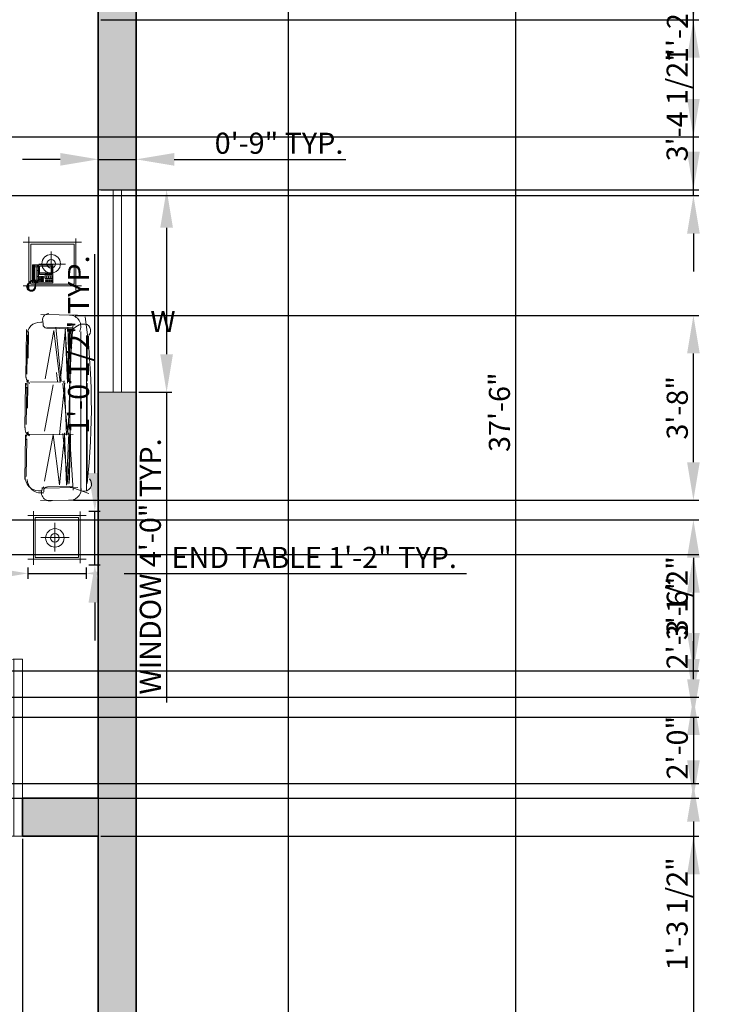
# Model space of a CAD drawing. Units: inches. Extents: x 2265 to 2807, y 1544 to 2401.
# Tile 8 of 9: x 2643 to 2807, y 1890 to 2124. Entities that reach past the tile are written whole.
import ezdxf

# ---------------------------------------------------------------- set-up
doc = ezdxf.new("R2010")
doc.units = ezdxf.units.IN
for name, color, linetype, lineweight in [('A-ANNO-DIMS', 2, 'Continuous', 18), ('A-ANNO-TEXT', 7, 'Continuous', 18), ('A-DOOR', 3, 'Continuous', 18), ('A-GLAZ', 4, 'Continuous', 18), ('A-WALL', 7, 'Continuous', 35), ('A-WALL-PATT', 18, 'Continuous', 13), ('C-PROP', 7, 'Continuous', 25), ('Furniture', 161, 'Continuous', 15)]:
    doc.layers.add(name, color=color, linetype=linetype, lineweight=lineweight)
doc.styles.add('ARIAL', font='times.ttf', dxfattribs={"height": 5})
doc.styles.get("Standard").update_dxf_attribs({"font": 'arial.ttf', "height": 5})
doc.dimstyles.new('ISO-25', dxfattribs={"dimtxt": 5, "dimasz": 9, "dimexe": 1.25, "dimexo": 0.625, "dimtad": 1, "dimlunit": 3, "dimtxsty": 'Standard', "dimcen": 2.5, "dimadec": 0, "dimazin": 0, "dimtfac": 1, "dimtmove": 0, "dimatfit": 3, "dimfxl": 1, "dimarcsym": 0})

# ---------------------------------------------------------------- blocks, each defined once
blk = doc.blocks.new('*D6')
at = {"layer": 'A-ANNO-DIMS', "color": 0, "lineweight": -2, "transparency": 16777216}
for p, q in [((2707.73, 2255.73), (2762.29, 2255.73)), ((2761.04, 2246.73), (2761.04, 1814.73)), ((2707.73, 1805.73), (2762.29, 1805.73))]:
    blk.add_line(p, q, dxfattribs=at)
at = {"layer": 'A-ANNO-DIMS', "color": 0, "lineweight": 100, "transparency": 16777216}
for points in [[(2759.54, 2246.73), (2762.54, 2246.73), (2761.04, 2255.73)], [(2759.54, 1814.73), (2762.54, 1814.73), (2761.04, 1805.73)]]:
    blk.add_solid(points, dxfattribs=at)
at = {"layer": 'Defpoints', "color": 0, "lineweight": 100, "transparency": 16777216}
for p in [(2707.1, 2255.73), (2707.1, 1805.73), (2761.04, 1805.73)]:
    blk.add_point(p, dxfattribs=at)
at = {"layer": 'A-ANNO-DIMS', "color": 0, "transparency": 16777216, "insert": (2757.86, 2030.73), "char_height": 5, "attachment_point": 5, "rotation": 90}
blk.add_mtext('37\'-6"', dxfattribs=at)
blk = doc.blocks.new('GLAZING-48IN')
for p, q in [((48, 9), (0, 9)), ((0, 5.5), (48, 5.5)), ((0, 5.5), (48, 5.5)), ((0, 3.5), (48, 3.5)), ((0, 0), (48, 0))]:
    blk.add_line(p, q)
blk = doc.blocks.new('END-TABLE')
for p, q in [((1.35, 12.69), (1.35, 0)), ((12.46, 0.37), (12.46, 12.6)), ((13.82, 11.62), (0, 11.62)), ((1.77, 11.2), (1.77, 1.7)), ((12.04, 11.2), (1.77, 11.2)), ((12.04, 1.7), (12.04, 11.2)), ((0, 1.28), (13.82, 1.28)), ((1.77, 1.7), (12.04, 1.7))]:
    blk.add_line(p, q)
blk = doc.blocks.new('DOOR-SWING-42IN')
for p, q in [((40, 41.95), (40, 0)), ((42, 0), (0, 0))]:
    blk.add_line(p, q)
blk.add_arc((42, 0), 42, 90, 180)
blk = doc.blocks.new('*D19')
at = {"layer": 'A-ANNO-DIMS', "color": 0, "lineweight": -2, "transparency": 16777216}
for p, q in [((2671.73, 2083.44), (2679.55, 2083.44)), ((2678.3, 2074.44), (2678.3, 2044.44)), ((2671.73, 2035.44), (2679.55, 2035.44)), ((2678.3, 2035.44), (2678.3, 1961.91))]:
    blk.add_line(p, q, dxfattribs=at)
at = {"layer": 'A-ANNO-DIMS', "color": 0, "lineweight": 100, "transparency": 16777216}
for points in [[(2676.8, 2074.44), (2679.8, 2074.44), (2678.3, 2083.44)], [(2676.8, 2044.44), (2679.8, 2044.44), (2678.3, 2035.44)]]:
    blk.add_solid(points, dxfattribs=at)
at = {"layer": 'Defpoints', "color": 0, "lineweight": 100, "transparency": 16777216}
for p in [(2671.1, 2083.44), (2671.1, 2035.44), (2678.3, 2035.44)]:
    blk.add_point(p, dxfattribs=at)
at = {"layer": 'A-ANNO-DIMS', "color": 0, "transparency": 16777216, "insert": (2675.09, 1994.17), "char_height": 5, "attachment_point": 5, "rotation": 90}
blk.add_mtext('WINDOW 4\'-0" TYP.', dxfattribs=at)
blk = doc.blocks.new('*D20')
at = {"layer": 'A-ANNO-DIMS', "color": 0, "lineweight": -2, "transparency": 16777216}
for p, q in [((2653.1, 2090.64), (2644.1, 2090.64)), ((2662.1, 2084.06), (2662.1, 2091.89)), ((2662.1, 2090.64), (2671.1, 2090.64)), ((2671.1, 2084.06), (2671.1, 2091.89)), ((2680.1, 2090.64), (2720.83, 2090.64))]:
    blk.add_line(p, q, dxfattribs=at)
at = {"layer": 'A-ANNO-DIMS', "color": 0, "lineweight": 100, "transparency": 16777216}
for points in [[(2653.1, 2092.14), (2653.1, 2089.14), (2662.1, 2090.64)], [(2680.1, 2092.14), (2680.1, 2089.14), (2671.1, 2090.64)]]:
    blk.add_solid(points, dxfattribs=at)
at = {"layer": 'Defpoints', "color": 0, "lineweight": 100, "transparency": 16777216}
for p in [(2671.1, 2090.64), (2662.1, 2083.44), (2671.1, 2083.44)]:
    blk.add_point(p, dxfattribs=at)
at = {"layer": 'A-ANNO-DIMS', "color": 0, "transparency": 16777216, "insert": (2704.96, 2093.81), "char_height": 5, "attachment_point": 5}
blk.add_mtext('0\'-9" TYP.', dxfattribs=at)
blk = doc.blocks.new('*D29')
at = {"layer": 'A-ANNO-DIMS', "color": 0, "lineweight": -2, "transparency": 16777216}
for p, q in [((2645.38, 1993.96), (2645.38, 1991.27)), ((2659.2, 1993.96), (2659.2, 1991.27)), ((2636.38, 1992.52), (2627.38, 1992.52)), ((2645.38, 1992.52), (2659.2, 1992.52)), ((2668.2, 1992.52), (2749.43, 1992.52))]:
    blk.add_line(p, q, dxfattribs=at)
at = {"layer": 'A-ANNO-DIMS', "color": 0, "lineweight": 100, "transparency": 16777216}
for points in [[(2636.38, 1994.02), (2636.38, 1991.02), (2645.38, 1992.52)], [(2668.2, 1994.02), (2668.2, 1991.02), (2659.2, 1992.52)]]:
    blk.add_solid(points, dxfattribs=at)
at = {"layer": 'Defpoints', "color": 0, "lineweight": 100, "transparency": 16777216}
for p in [(2645.38, 1994.59), (2659.2, 1994.59), (2659.2, 1992.52)]:
    blk.add_point(p, dxfattribs=at)
at = {"layer": 'A-ANNO-DIMS', "color": 0, "transparency": 16777216, "insert": (2713.31, 1995.65), "char_height": 5, "attachment_point": 5}
blk.add_mtext('END TABLE 1\'-2" TYP.', dxfattribs=at)
blk = doc.blocks.new('*D30')
at = {"layer": 'A-ANNO-DIMS', "color": 0, "lineweight": -2, "transparency": 16777216}
for p, q in [((2661.28, 2016.28), (2661.28, 2068.19)), ((2659.83, 2007.28), (2662.53, 2007.28)), ((2661.28, 1994.59), (2661.28, 2007.28)), ((2659.83, 1994.59), (2662.53, 1994.59)), ((2661.28, 1985.59), (2661.28, 1976.59))]:
    blk.add_line(p, q, dxfattribs=at)
at = {"layer": 'A-ANNO-DIMS', "color": 0, "lineweight": 100, "transparency": 16777216}
for points in [[(2659.78, 2016.28), (2662.78, 2016.28), (2661.28, 2007.28)], [(2659.78, 1985.59), (2662.78, 1985.59), (2661.28, 1994.59)]]:
    blk.add_solid(points, dxfattribs=at)
at = {"layer": 'Defpoints', "color": 0, "lineweight": 100, "transparency": 16777216}
for p in [(2659.2, 2007.28), (2661.28, 2007.28), (2659.2, 1994.59)]:
    blk.add_point(p, dxfattribs=at)
at = {"layer": 'A-ANNO-DIMS', "color": 0, "transparency": 16777216, "insert": (2658.07, 2046.74), "char_height": 5, "attachment_point": 5, "rotation": 90}
blk.add_mtext('1\'-0 1/2" TYP.', dxfattribs=at)
blk = doc.blocks.new('*D35')
at = {"layer": 'A-ANNO-DIMS', "color": 0, "lineweight": -2, "transparency": 16777216}
for p, q in [((2581.1, 2123.11), (2581.1, 1546.93)), ((2662.1, 2123.11), (2662.1, 1546.93)), ((2590.1, 1548.18), (2653.1, 1548.18))]:
    blk.add_line(p, q, dxfattribs=at)
at = {"layer": 'A-ANNO-DIMS', "color": 0, "lineweight": 100, "transparency": 16777216}
for points in [[(2590.1, 1549.68), (2590.1, 1546.68), (2581.1, 1548.18)], [(2653.1, 1549.68), (2653.1, 1546.68), (2662.1, 1548.18)]]:
    blk.add_solid(points, dxfattribs=at)
at = {"layer": 'Defpoints', "color": 0, "lineweight": 100, "transparency": 16777216}
for p in [(2581.1, 2123.73), (2662.1, 2123.73), (2662.1, 1548.18)]:
    blk.add_point(p, dxfattribs=at)
at = {"layer": 'A-ANNO-DIMS', "color": 0, "transparency": 16777216, "insert": (2621.6, 1551.36), "char_height": 5, "attachment_point": 5}
blk.add_mtext('6\'-9"', dxfattribs=at)
blk = doc.blocks.new('*D36')
at = {"layer": 'A-ANNO-DIMS', "color": 0, "lineweight": -2, "transparency": 16777216}
for p, q in [((2662.73, 2246.73), (2804.46, 2246.73)), ((2803.21, 2237.73), (2803.21, 2132.73)), ((2662.73, 2123.73), (2804.46, 2123.73))]:
    blk.add_line(p, q, dxfattribs=at)
at = {"layer": 'A-ANNO-DIMS', "color": 0, "lineweight": 100, "transparency": 16777216}
for points in [[(2801.71, 2237.73), (2804.71, 2237.73), (2803.21, 2246.73)], [(2801.71, 2132.73), (2804.71, 2132.73), (2803.21, 2123.73)]]:
    blk.add_solid(points, dxfattribs=at)
at = {"layer": 'Defpoints', "color": 0, "lineweight": 100, "transparency": 16777216}
for p in [(2662.1, 2246.73), (2662.1, 2123.73), (2803.21, 2123.73)]:
    blk.add_point(p, dxfattribs=at)
at = {"layer": 'A-ANNO-DIMS', "color": 0, "transparency": 16777216, "insert": (2800.03, 2185.23), "char_height": 5, "attachment_point": 5, "rotation": 90}
blk.add_mtext('10\'-3"', dxfattribs=at)
blk = doc.blocks.new('*D39')
at = {"layer": 'A-ANNO-DIMS', "color": 0, "lineweight": -2, "transparency": 16777216}
for p, q in [((2644.1, 1929.61), (2644.1, 1546.93)), ((2662.1, 1929.61), (2662.1, 1546.93)), ((2635.1, 1548.18), (2626.1, 1548.18)), ((2644.1, 1548.18), (2662.1, 1548.18)), ((2671.1, 1548.18), (2680.1, 1548.18))]:
    blk.add_line(p, q, dxfattribs=at)
at = {"layer": 'A-ANNO-DIMS', "color": 0, "lineweight": 100, "transparency": 16777216}
for points in [[(2635.1, 1549.68), (2635.1, 1546.68), (2644.1, 1548.18)], [(2671.1, 1549.68), (2671.1, 1546.68), (2662.1, 1548.18)]]:
    blk.add_solid(points, dxfattribs=at)
at = {"layer": 'Defpoints', "color": 0, "lineweight": 100, "transparency": 16777216}
for p in [(2644.1, 1930.23), (2662.1, 1930.23), (2662.1, 1548.18)]:
    blk.add_point(p, dxfattribs=at)
at = {"layer": 'A-ANNO-DIMS', "color": 0, "transparency": 16777216, "insert": (2653.1, 1551.36), "char_height": 5, "attachment_point": 5}
blk.add_mtext('1\'-6"', dxfattribs=at)
blk = doc.blocks.new('*D41')
at = {"layer": 'A-ANNO-DIMS', "color": 0, "lineweight": -2, "transparency": 16777216}
for p, q in [((2392.73, 2005.23), (2804.46, 2005.23)), ((2803.21, 1996.23), (2803.21, 1972.23)), ((2392.73, 1963.23), (2804.46, 1963.23))]:
    blk.add_line(p, q, dxfattribs=at)
at = {"layer": 'A-ANNO-DIMS', "color": 0, "lineweight": 100, "transparency": 16777216}
for points in [[(2801.71, 1996.23), (2804.71, 1996.23), (2803.21, 2005.23)], [(2801.71, 1972.23), (2804.71, 1972.23), (2803.21, 1963.23)]]:
    blk.add_solid(points, dxfattribs=at)
at = {"layer": 'Defpoints', "color": 0, "lineweight": 100, "transparency": 16777216}
for p in [(2392.1, 2005.23), (2392.1, 1963.23), (2803.21, 1963.23)]:
    blk.add_point(p, dxfattribs=at)
at = {"layer": 'A-ANNO-DIMS', "color": 0, "transparency": 16777216, "insert": (2800.03, 1984.23), "char_height": 5, "attachment_point": 5, "rotation": 90}
blk.add_mtext('3\'-6"', dxfattribs=at)
blk = doc.blocks.new('*D42')
at = {"layer": 'A-ANNO-DIMS', "color": 0, "lineweight": -2, "transparency": 16777216}
for p, q in [((2464.73, 1963.23), (2804.46, 1963.23)), ((2803.21, 1954.23), (2803.21, 1948.23)), ((2464.73, 1939.23), (2804.46, 1939.23))]:
    blk.add_line(p, q, dxfattribs=at)
at = {"layer": 'A-ANNO-DIMS', "color": 0, "lineweight": 100, "transparency": 16777216}
for points in [[(2801.71, 1954.23), (2804.71, 1954.23), (2803.21, 1963.23)], [(2801.71, 1948.23), (2804.71, 1948.23), (2803.21, 1939.23)]]:
    blk.add_solid(points, dxfattribs=at)
at = {"layer": 'Defpoints', "color": 0, "lineweight": 100, "transparency": 16777216}
for p in [(2464.1, 1963.23), (2464.1, 1939.23), (2803.21, 1939.23)]:
    blk.add_point(p, dxfattribs=at)
at = {"layer": 'A-ANNO-DIMS', "color": 0, "transparency": 16777216, "insert": (2800.03, 1951.23), "char_height": 5, "attachment_point": 5, "rotation": 90}
blk.add_mtext('2\'-0"', dxfattribs=at)
blk = doc.blocks.new('*D46')
at = {"layer": 'A-ANNO-DIMS', "color": 0, "lineweight": -2, "transparency": 16777216}
for p, q in [((2803.21, 2104.95), (2803.21, 2128.02)), ((2381.23, 2095.95), (2804.46, 2095.95)), ((2803.21, 2082.06), (2803.21, 2095.95)), ((2381.23, 2082.06), (2804.46, 2082.06)), ((2803.21, 2073.06), (2803.21, 2064.06))]:
    blk.add_line(p, q, dxfattribs=at)
at = {"layer": 'A-ANNO-DIMS', "color": 0, "lineweight": 100, "transparency": 16777216}
for points in [[(2801.71, 2104.95), (2804.71, 2104.95), (2803.21, 2095.95)], [(2801.71, 2073.06), (2804.71, 2073.06), (2803.21, 2082.06)]]:
    blk.add_solid(points, dxfattribs=at)
at = {"layer": 'Defpoints', "color": 0, "lineweight": 100, "transparency": 16777216}
for p in [(2380.61, 2095.95), (2803.21, 2095.95), (2380.61, 2082.06)]:
    blk.add_point(p, dxfattribs=at)
at = {"layer": 'A-ANNO-DIMS', "color": 0, "transparency": 16777216, "insert": (2800.07, 2120.99), "char_height": 5, "attachment_point": 5, "rotation": 90}
blk.add_mtext('1\'-2"', dxfattribs=at)
blk = doc.blocks.new('*D53')
at = {"layer": 'A-ANNO-DIMS', "color": 0, "lineweight": -2, "transparency": 16777216}
for p, q in [((2662.73, 1930.23), (2804.46, 1930.23)), ((2803.21, 1921.23), (2803.21, 1823.73)), ((2662.73, 1814.73), (2804.46, 1814.73))]:
    blk.add_line(p, q, dxfattribs=at)
at = {"layer": 'A-ANNO-DIMS', "color": 0, "lineweight": 100, "transparency": 16777216}
for points in [[(2801.71, 1921.23), (2804.71, 1921.23), (2803.21, 1930.23)], [(2801.71, 1823.73), (2804.71, 1823.73), (2803.21, 1814.73)]]:
    blk.add_solid(points, dxfattribs=at)
at = {"layer": 'Defpoints', "color": 0, "lineweight": 100, "transparency": 16777216}
for p in [(2662.1, 1930.23), (2662.1, 1814.73), (2803.21, 1814.73)]:
    blk.add_point(p, dxfattribs=at)
at = {"layer": 'A-ANNO-DIMS', "color": 0, "transparency": 16777216, "insert": (2800, 1872.48), "char_height": 5, "attachment_point": 5, "rotation": 90}
blk.add_mtext('9\'-7 1/2"', dxfattribs=at)
blk = doc.blocks.new('*D58')
at = {"layer": 'A-ANNO-DIMS', "color": 0, "lineweight": -2, "transparency": 16777216}
for p, q in [((2662.73, 2123.73), (2804.46, 2123.73)), ((2803.21, 2092.44), (2803.21, 2114.73)), ((2662.73, 2083.44), (2804.46, 2083.44))]:
    blk.add_line(p, q, dxfattribs=at)
at = {"layer": 'A-ANNO-DIMS', "color": 0, "lineweight": 100, "transparency": 16777216}
for points in [[(2801.71, 2114.73), (2804.71, 2114.73), (2803.21, 2123.73)], [(2801.71, 2092.44), (2804.71, 2092.44), (2803.21, 2083.44)]]:
    blk.add_solid(points, dxfattribs=at)
at = {"layer": 'Defpoints', "color": 0, "lineweight": 100, "transparency": 16777216}
for p in [(2662.1, 2123.73), (2803.21, 2123.73), (2662.1, 2083.44)]:
    blk.add_point(p, dxfattribs=at)
at = {"layer": 'A-ANNO-DIMS', "color": 0, "transparency": 16777216, "insert": (2800, 2103.58), "char_height": 5, "attachment_point": 5, "rotation": 90}
blk.add_mtext('3\'-4 1/2"', dxfattribs=at)
blk = doc.blocks.new('*D61')
at = {"layer": 'A-ANNO-DIMS', "color": 0, "lineweight": -2, "transparency": 16777216}
for p, q in [((2803.21, 1967.45), (2803.21, 1976.45)), ((2444.67, 1958.45), (2804.46, 1958.45)), ((2803.21, 1958.45), (2803.21, 1942.7)), ((2444.67, 1942.7), (2804.46, 1942.7)), ((2803.21, 1933.7), (2803.21, 1898.98))]:
    blk.add_line(p, q, dxfattribs=at)
at = {"layer": 'A-ANNO-DIMS', "color": 0, "lineweight": 100, "transparency": 16777216}
for points in [[(2801.71, 1967.45), (2804.71, 1967.45), (2803.21, 1958.45)], [(2801.71, 1933.7), (2804.71, 1933.7), (2803.21, 1942.7)]]:
    blk.add_solid(points, dxfattribs=at)
at = {"layer": 'Defpoints', "color": 0, "lineweight": 100, "transparency": 16777216}
for p in [(2444.05, 1958.45), (2444.05, 1942.7), (2803.21, 1942.7)]:
    blk.add_point(p, dxfattribs=at)
at = {"layer": 'A-ANNO-DIMS', "color": 0, "transparency": 16777216, "insert": (2800, 1911.84), "char_height": 5, "attachment_point": 5, "rotation": 90}
blk.add_mtext('1\'-3 1/2"', dxfattribs=at)
blk = doc.blocks.new('*D64')
at = {"layer": 'A-ANNO-DIMS', "color": 0, "lineweight": -2, "transparency": 16777216}
for p, q in [((2521.03, 1996.97), (2804.46, 1996.97)), ((2803.21, 1978.41), (2803.21, 1987.97)), ((2521.03, 1969.41), (2804.46, 1969.41))]:
    blk.add_line(p, q, dxfattribs=at)
at = {"layer": 'A-ANNO-DIMS', "color": 0, "lineweight": 100, "transparency": 16777216}
for points in [[(2801.71, 1987.97), (2804.71, 1987.97), (2803.21, 1996.97)], [(2801.71, 1978.41), (2804.71, 1978.41), (2803.21, 1969.41)]]:
    blk.add_solid(points, dxfattribs=at)
at = {"layer": 'Defpoints', "color": 0, "lineweight": 100, "transparency": 16777216}
for p in [(2520.4, 1996.97), (2803.21, 1996.97), (2520.4, 1969.41)]:
    blk.add_point(p, dxfattribs=at)
at = {"layer": 'A-ANNO-DIMS', "color": 0, "transparency": 16777216, "insert": (2800, 1983.19), "char_height": 5, "attachment_point": 5, "rotation": 90}
blk.add_mtext('2\'-3 1/2"', dxfattribs=at)
blk = doc.blocks.new('*D65')
at = {"layer": 'A-ANNO-DIMS', "color": 0, "lineweight": -2, "transparency": 16777216}
for p, q in [((2656.62, 2053.64), (2804.46, 2053.64)), ((2803.21, 2018.88), (2803.21, 2044.64)), ((2656.22, 2009.88), (2804.46, 2009.88))]:
    blk.add_line(p, q, dxfattribs=at)
at = {"layer": 'A-ANNO-DIMS', "color": 0, "lineweight": 100, "transparency": 16777216}
for points in [[(2801.71, 2044.64), (2804.71, 2044.64), (2803.21, 2053.64)], [(2801.71, 2018.88), (2804.71, 2018.88), (2803.21, 2009.88)]]:
    blk.add_solid(points, dxfattribs=at)
at = {"layer": 'Defpoints', "color": 0, "lineweight": 100, "transparency": 16777216}
for p in [(2655.99, 2053.64), (2803.21, 2053.64), (2655.59, 2009.88)]:
    blk.add_point(p, dxfattribs=at)
at = {"layer": 'A-ANNO-DIMS', "color": 0, "transparency": 16777216, "insert": (2800.03, 2031.76), "char_height": 5, "attachment_point": 5, "rotation": 90}
blk.add_mtext('3\'-8"', dxfattribs=at)

msp = doc.modelspace()

# ---------------------------------------------------------------- hatches: boundary and pattern name
at = {"layer": 'A-WALL-PATT'}
h = msp.add_hatch(color=256, dxfattribs=at)
h.dxf.hatch_style = 1
h.paths.add_polyline_path([(2416.101, 2255.733), (2359.101, 2255.733), (2359.101, 2205.483), (2368.101, 2205.483), (2368.101, 2246.733), (2416.101, 2246.733)])
h.paths.add_polyline_path([(2528.601, 2255.733), (2452.101, 2255.733), (2452.101, 2246.733), (2487.251, 2246.733), (2500.101, 2246.733), (2500.101, 2168.733), (2504.601, 2168.733), (2504.601, 2170.233), (2525.601, 2170.233), (2525.601, 2174.733), (2504.601, 2174.733), (2504.601, 2246.733), (2528.601, 2246.733)])
h.paths.add_polyline_path([(2603.601, 2255.733), (2552.601, 2255.733), (2552.601, 2246.733), (2576.601, 2246.733), (2576.601, 2174.733), (2555.601, 2174.733), (2555.601, 2170.233), (2576.601, 2170.233), (2576.601, 2123.733), (2581.101, 2123.733), (2581.101, 2246.733), (2603.601, 2246.733)])
h.paths.add_polyline_path([(2671.101, 2255.733), (2639.601, 2255.733), (2639.601, 2246.733), (2662.101, 2246.733), (2662.101, 2083.435), (2671.101, 2083.435)])
h.paths.add_polyline_path([(2671.101, 2035.435), (2662.101, 2035.435), (2662.101, 1939.233), (2644.101, 1939.233), (2644.101, 1930.233), (2662.101, 1930.233), (2662.101, 1814.733), (2644.101, 1814.733), (2644.101, 1805.733), (2671.101, 1805.733)])
h.paths.add_polyline_path([(2368.101, 1930.233), (2511.351, 1930.233), (2511.351, 1939.233), (2468.601, 1939.233), (2468.601, 2032.233), (2464.101, 2032.233), (2464.101, 1939.233), (2368.101, 1939.233), (2368.101, 1995.884), (2359.101, 1995.884), (2359.101, 1805.733), (2602.101, 1805.733), (2602.101, 1814.733), (2368.101, 1814.733)])
h.paths.add_polyline_path([(2368.101, 2071.233), (2464.101, 2071.233), (2464.101, 2062.233), (2468.601, 2062.233), (2468.601, 2123.733), (2504.601, 2123.733), (2504.601, 2132.733), (2500.101, 2132.733), (2500.101, 2128.233), (2455.101, 2128.233), (2455.101, 2123.733), (2464.101, 2123.733), (2464.101, 2075.733), (2368.101, 2075.733), (2368.101, 2087.733), (2359.101, 2087.733), (2359.101, 2031.884), (2368.101, 2031.884)])
h.paths.add_polyline_path([(2368.101, 2169.483), (2359.101, 2169.483), (2359.101, 2111.733), (2368.101, 2111.733), (2368.101, 2123.733), (2425.101, 2123.733), (2425.101, 2128.233), (2368.101, 2128.233)])

# ---------------------------------------------------------------- linework, layer by layer
at = {"layer": 'A-DOOR'}
msp.add_line((2644.101, 1972.233), (2644.101, 1930.233), dxfattribs=at)
at = {"layer": 'A-GLAZ'}
for p, q in [((2671.101, 2083.435), (2662.101, 2083.435)), ((2662.101, 2035.435), (2671.101, 2035.435))]:
    msp.add_line(p, q, dxfattribs=at)
at = {"layer": 'A-WALL'}
for p, q in [((2671.101, 2255.733), (2671.101, 1805.733)), ((2662.101, 2246.733), (2662.101, 1939.233)), ((2662.101, 1939.233), (2644.101, 1939.233)), ((2644.101, 1939.233), (2644.101, 1930.233)), ((2662.101, 1930.233), (2644.101, 1930.233)), ((2662.101, 1930.233), (2662.101, 1814.733))]:
    msp.add_line(p, q, dxfattribs=at)
at = {"layer": 'C-PROP'}
msp.add_line((2707.101, 2255.733), (2707.101, 1805.733), dxfattribs=at)
at = {"layer": 'Furniture'}
for p, q in [((2650.929, 2068.806), (2650.929, 2063.417)), ((2646.557, 2065.646), (2646.497, 2065.586)), ((2646.497, 2065.586), (2646.497, 2061.443)), ((2651.301, 2065.646), (2646.557, 2065.646)), ((2646.888, 2065.556), (2646.738, 2065.406)), ((2646.738, 2065.406), (2646.738, 2061.803)), ((2646.828, 2065.466), (2646.798, 2065.345)), ((2646.798, 2065.345), (2647.068, 2065.075)), ((2646.798, 2065.345), (2646.798, 2064.535)), ((2646.948, 2065.526), (2646.828, 2065.466)), ((2647.788, 2065.556), (2646.888, 2065.556)), ((2647.098, 2065.135), (2646.948, 2065.526)), ((2647.668, 2065.526), (2646.948, 2065.526)), ((2647.068, 2065.075), (2647.098, 2065.135)), ((2647.068, 2063.724), (2647.068, 2065.075)), ((2647.098, 2065.135), (2647.518, 2065.135)), ((2647.518, 2065.135), (2647.668, 2065.526)), ((2647.548, 2065.075), (2647.518, 2065.135)), ((2647.818, 2065.345), (2647.548, 2065.075)), ((2647.548, 2063.724), (2647.548, 2065.075)), ((2647.668, 2065.526), (2647.788, 2065.466)), ((2647.908, 2065.406), (2647.788, 2065.556)), ((2647.788, 2065.466), (2647.818, 2065.345)), ((2647.818, 2065.345), (2647.818, 2064.535)), ((2647.908, 2061.773), (2647.908, 2065.406)), ((2648.016, 2065.838), (2654.303, 2065.838)), ((2648.179, 2065.315), (2651.181, 2065.315)), ((2648.179, 2063.724), (2648.179, 2065.315)), ((2651.181, 2065.315), (2651.181, 2063.724)), ((2651.301, 2065.646), (2651.361, 2065.586)), ((2651.361, 2065.586), (2651.361, 2061.443)), ((2646.798, 2064.535), (2646.858, 2064.385)), ((2646.798, 2062.644), (2646.858, 2062.794)), ((2646.798, 2061.833), (2646.798, 2062.644)), ((2646.858, 2064.385), (2646.948, 2064.235)), ((2646.858, 2062.794), (2646.948, 2062.944)), ((2646.948, 2064.235), (2646.978, 2064.025)), ((2646.948, 2062.944), (2646.978, 2063.154)), ((2646.978, 2064.025), (2646.978, 2063.724)), ((2646.978, 2063.154), (2646.978, 2063.724)), ((2647.068, 2063.724), (2647.068, 2062.103)), ((2647.548, 2063.724), (2647.548, 2062.103)), ((2647.668, 2064.235), (2647.638, 2064.025)), ((2647.638, 2064.025), (2647.638, 2063.724)), ((2647.638, 2063.154), (2647.638, 2063.724)), ((2647.668, 2062.944), (2647.638, 2063.154)), ((2647.758, 2064.385), (2647.668, 2064.235)), ((2647.758, 2062.794), (2647.668, 2062.944)), ((2647.818, 2064.535), (2647.758, 2064.385)), ((2647.818, 2062.644), (2647.758, 2062.794)), ((2647.818, 2061.833), (2647.818, 2062.644)), ((2651.181, 2063.724), (2648.179, 2063.724)), ((2648.179, 2063.664), (2651.061, 2063.664)), ((2648.179, 2063.364), (2648.179, 2063.664)), ((2651.061, 2063.364), (2648.179, 2063.364)), ((2648.419, 2062.884), (2648.179, 2062.884)), ((2648.179, 2062.884), (2648.179, 2062.704)), ((2648.179, 2062.704), (2648.419, 2062.704)), ((2648.419, 2062.704), (2648.419, 2062.884)), ((2648.539, 2062.884), (2648.539, 2062.704)), ((2648.779, 2062.884), (2648.539, 2062.884)), ((2648.539, 2062.704), (2648.779, 2062.704)), ((2648.779, 2062.704), (2648.779, 2062.884)), ((2649.139, 2062.884), (2648.899, 2062.884)), ((2648.899, 2062.884), (2648.899, 2062.704)), ((2648.899, 2062.704), (2649.139, 2062.704)), ((2649.139, 2062.704), (2649.139, 2062.884)), ((2649.409, 2063.034), (2651.181, 2063.034)), ((2649.409, 2062.493), (2649.409, 2063.034)), ((2649.62, 2063.664), (2649.62, 2063.364)), ((2649.71, 2062.884), (2649.71, 2062.974)), ((2649.71, 2062.974), (2649.8, 2062.974)), ((2649.8, 2062.884), (2649.71, 2062.884)), ((2649.71, 2062.554), (2649.71, 2062.644)), ((2649.71, 2062.644), (2649.8, 2062.644)), ((2649.8, 2062.974), (2649.8, 2062.884)), ((2649.8, 2062.644), (2649.8, 2062.554)), ((2649.86, 2063.664), (2649.86, 2063.364)), ((2650.1, 2063.664), (2650.1, 2063.364)), ((2650.25, 2062.884), (2650.25, 2062.974)), ((2650.25, 2062.974), (2650.34, 2062.974)), ((2650.34, 2062.884), (2650.25, 2062.884)), ((2650.25, 2062.554), (2650.25, 2062.644)), ((2650.25, 2062.644), (2650.34, 2062.644)), ((2650.34, 2063.664), (2650.34, 2063.364)), ((2650.34, 2062.974), (2650.34, 2062.884)), ((2650.34, 2062.644), (2650.34, 2062.554)), ((2650.58, 2063.664), (2650.58, 2063.364)), ((2650.79, 2062.974), (2650.881, 2062.974)), ((2650.79, 2062.884), (2650.79, 2062.974)), ((2650.881, 2062.884), (2650.79, 2062.884)), ((2650.79, 2062.554), (2650.79, 2062.644)), ((2650.79, 2062.644), (2650.881, 2062.644)), ((2650.82, 2063.664), (2650.82, 2063.364)), ((2650.881, 2062.974), (2650.881, 2062.884)), ((2650.881, 2062.644), (2650.881, 2062.554)), ((2651.061, 2063.664), (2651.061, 2063.364)), ((2651.181, 2063.034), (2651.181, 2062.493)), ((2645.116, 2060.426), (2645.147, 2060.578)), ((2645.305, 2060.372), (2645.116, 2060.426)), ((2645.147, 2060.578), (2645.311, 2060.578)), ((2645.147, 2060.28), (2645.305, 2060.372)), ((2645.171, 2060.159), (2645.147, 2060.28)), ((2645.183, 2060.7), (2645.226, 2060.84)), ((2645.311, 2060.578), (2645.183, 2060.7)), ((2645.226, 2060.84), (2645.42, 2060.834)), ((2645.244, 2060.9), (2645.299, 2061.083)), ((2645.42, 2060.834), (2645.244, 2060.9)), ((2645.299, 2061.083), (2645.481, 2061.065)), ((2645.566, 2061.065), (2645.365, 2060.493)), ((2645.365, 2060.493), (2645.45, 2060.037)), ((2645.434, 2061.197), (2645.551, 2061.318)), ((2645.482, 2061.064), (2645.434, 2061.197)), ((2645.551, 2061.318), (2645.688, 2061.234)), ((2645.968, 2061.413), (2645.572, 2061.075)), ((2645.656, 2061.424), (2645.794, 2061.556)), ((2645.688, 2061.234), (2645.656, 2061.424)), ((2645.794, 2061.556), (2645.958, 2061.472)), ((2645.894, 2061.646), (2645.974, 2061.731)), ((2645.958, 2061.472), (2645.894, 2061.646)), ((2646.212, 2061.63), (2645.968, 2061.413)), ((2645.974, 2061.731), (2646.048, 2061.673)), ((2646.005, 2061.763), (2646.058, 2061.816)), ((2646.048, 2061.673), (2646.005, 2061.763)), ((2646.058, 2061.816), (2646.169, 2061.773)), ((2646.148, 2061.694), (2646.212, 2061.63)), ((2646.212, 2061.689), (2646.148, 2061.694)), ((2646.169, 2061.773), (2646.233, 2061.831)), ((2646.243, 2061.731), (2646.212, 2061.689)), ((2646.233, 2061.831), (2646.317, 2061.916)), ((2646.365, 2061.826), (2646.243, 2061.731)), ((2646.317, 2061.916), (2646.497, 2061.983)), ((2646.497, 2061.863), (2646.365, 2061.826)), ((2646.497, 2061.443), (2646.557, 2061.383)), ((2646.557, 2061.383), (2647.204, 2061.383)), ((2646.738, 2061.803), (2646.888, 2061.623)), ((2646.798, 2061.833), (2647.068, 2062.103)), ((2646.828, 2061.713), (2646.798, 2061.833)), ((2646.948, 2061.653), (2646.828, 2061.713)), ((2646.888, 2061.623), (2647.239, 2061.623)), ((2647.098, 2062.043), (2646.948, 2061.653)), ((2647.241, 2061.653), (2646.948, 2061.653)), ((2646.988, 2060.116), (2647.018, 2060.499)), ((2646.994, 2060.639), (2647.103, 2060.718)), ((2647.018, 2060.499), (2646.994, 2060.639)), ((2647.068, 2062.103), (2647.098, 2062.043)), ((2647.255, 2060.487), (2647.079, 2060.457)), ((2647.079, 2060.457), (2647.249, 2060.353)), ((2647.097, 2060.876), (2647.115, 2061.022)), ((2647.103, 2060.718), (2647.097, 2060.876)), ((2647.098, 2062.043), (2647.518, 2062.043)), ((2647.115, 2061.022), (2647.188, 2061.308)), ((2647.194, 2060.736), (2647.176, 2060.7)), ((2647.176, 2060.7), (2647.243, 2060.633)), ((2647.188, 2061.308), (2647.231, 2061.502)), ((2647.261, 2061.18), (2647.188, 2060.894)), ((2647.188, 2060.894), (2647.194, 2060.736)), ((2647.231, 2061.502), (2647.248, 2061.743)), ((2647.249, 2060.353), (2647.237, 2060.189)), ((2647.243, 2060.633), (2647.255, 2060.487)), ((2647.248, 2061.743), (2647.338, 2061.743)), ((2647.334, 2061.484), (2647.261, 2061.18)), ((2647.31, 2061.383), (2651.301, 2061.383)), ((2647.338, 2061.743), (2647.334, 2061.484)), ((2647.336, 2061.623), (2647.758, 2061.623)), ((2647.668, 2061.653), (2647.337, 2061.653)), ((2647.548, 2062.103), (2647.518, 2062.043)), ((2647.518, 2062.043), (2647.668, 2061.653)), ((2647.818, 2061.833), (2647.548, 2062.103)), ((2647.668, 2061.653), (2647.788, 2061.713)), ((2647.758, 2061.623), (2647.908, 2061.773)), ((2647.788, 2061.713), (2647.818, 2061.833)), ((2648.179, 2062.554), (2648.179, 2062.373)), ((2648.419, 2062.554), (2648.179, 2062.554)), ((2648.179, 2062.373), (2648.419, 2062.373)), ((2648.419, 2062.223), (2648.179, 2062.223)), ((2648.179, 2062.223), (2648.179, 2062.043)), ((2648.179, 2062.043), (2648.419, 2062.043)), ((2648.419, 2061.863), (2648.179, 2061.863)), ((2648.179, 2061.863), (2648.179, 2061.683)), ((2648.179, 2061.683), (2648.419, 2061.683)), ((2648.419, 2062.373), (2648.419, 2062.554)), ((2648.419, 2062.043), (2648.419, 2062.223)), ((2648.419, 2061.683), (2648.419, 2061.863)), ((2648.539, 2062.554), (2648.539, 2062.373)), ((2648.779, 2062.554), (2648.539, 2062.554)), ((2648.539, 2062.373), (2648.779, 2062.373)), ((2648.779, 2062.193), (2648.539, 2062.193)), ((2648.539, 2062.193), (2648.539, 2062.013)), ((2648.539, 2062.013), (2648.779, 2062.013)), ((2648.779, 2061.863), (2648.539, 2061.863)), ((2648.539, 2061.863), (2648.539, 2061.683)), ((2648.539, 2061.683), (2648.779, 2061.683)), ((2648.779, 2062.373), (2648.779, 2062.554)), ((2648.779, 2062.013), (2648.779, 2062.193)), ((2648.779, 2061.683), (2648.779, 2061.863)), ((2648.899, 2062.554), (2648.899, 2062.373)), ((2649.139, 2062.554), (2648.899, 2062.554)), ((2648.899, 2062.373), (2649.139, 2062.373)), ((2649.139, 2062.193), (2648.899, 2062.193)), ((2648.899, 2062.193), (2648.899, 2062.013)), ((2648.899, 2062.013), (2649.139, 2062.013)), ((2649.139, 2061.863), (2648.899, 2061.863)), ((2648.899, 2061.863), (2648.899, 2061.683)), ((2648.899, 2061.683), (2649.139, 2061.683)), ((2649.139, 2062.373), (2649.139, 2062.554)), ((2649.139, 2062.013), (2649.139, 2062.193)), ((2649.139, 2061.683), (2649.139, 2061.863)), ((2651.181, 2062.493), (2649.409, 2062.493)), ((2649.59, 2062.223), (2649.59, 2062.343)), ((2649.59, 2062.343), (2649.89, 2062.343)), ((2649.89, 2062.223), (2649.59, 2062.223)), ((2649.89, 2061.893), (2649.59, 2061.893)), ((2649.59, 2061.893), (2649.59, 2061.713)), ((2649.59, 2061.713), (2649.89, 2061.713)), ((2649.8, 2062.554), (2649.71, 2062.554)), ((2649.89, 2062.343), (2649.89, 2062.223)), ((2649.89, 2061.713), (2649.89, 2061.893)), ((2650.01, 2062.343), (2650.31, 2062.343)), ((2650.01, 2062.223), (2650.01, 2062.343)), ((2650.31, 2062.223), (2650.01, 2062.223)), ((2650.01, 2061.893), (2650.01, 2061.713)), ((2650.31, 2061.893), (2650.01, 2061.893)), ((2650.01, 2061.713), (2650.31, 2061.713)), ((2650.34, 2062.554), (2650.25, 2062.554)), ((2650.31, 2062.343), (2650.31, 2062.223)), ((2650.31, 2061.713), (2650.31, 2061.893)), ((2650.43, 2062.343), (2650.73, 2062.343)), ((2650.43, 2062.223), (2650.43, 2062.343)), ((2650.73, 2062.223), (2650.43, 2062.223)), ((2650.43, 2061.893), (2650.43, 2061.713)), ((2650.73, 2061.893), (2650.43, 2061.893)), ((2650.43, 2061.713), (2650.73, 2061.713)), ((2650.73, 2062.343), (2650.73, 2062.223)), ((2650.73, 2061.713), (2650.73, 2061.893)), ((2650.881, 2062.554), (2650.79, 2062.554)), ((2650.85, 2062.343), (2651.151, 2062.343)), ((2650.85, 2062.223), (2650.85, 2062.343)), ((2651.151, 2062.223), (2650.85, 2062.223)), ((2650.85, 2061.893), (2650.85, 2061.713)), ((2651.151, 2061.893), (2650.85, 2061.893)), ((2650.85, 2061.713), (2651.151, 2061.713)), ((2651.151, 2062.343), (2651.151, 2062.223)), ((2651.151, 2061.713), (2651.151, 2061.893)), ((2651.361, 2061.443), (2651.301, 2061.383)), ((2645.359, 2060.165), (2645.171, 2060.159)), ((2645.213, 2060.001), (2645.359, 2060.165)), ((2645.262, 2059.879), (2645.213, 2060.001)), ((2645.438, 2059.934), (2645.262, 2059.879)), ((2645.353, 2059.77), (2645.438, 2059.934)), ((2645.432, 2059.697), (2645.353, 2059.77)), ((2645.602, 2059.77), (2645.432, 2059.697)), ((2645.45, 2060.037), (2645.718, 2059.776)), ((2645.529, 2059.606), (2645.602, 2059.77)), ((2645.627, 2059.52), (2645.529, 2059.606)), ((2645.754, 2059.679), (2645.627, 2059.52)), ((2645.718, 2059.776), (2646.07, 2059.624)), ((2645.736, 2059.496), (2645.754, 2059.679)), ((2645.833, 2059.448), (2645.736, 2059.496)), ((2645.973, 2059.569), (2645.833, 2059.448)), ((2645.979, 2059.405), (2645.973, 2059.569)), ((2646.094, 2059.375), (2645.979, 2059.405)), ((2646.07, 2059.624), (2646.435, 2059.654)), ((2646.161, 2059.569), (2646.094, 2059.375)), ((2646.204, 2059.393), (2646.161, 2059.569)), ((2646.307, 2059.405), (2646.204, 2059.393)), ((2646.38, 2059.569), (2646.307, 2059.405)), ((2646.459, 2059.405), (2646.38, 2059.569)), ((2646.435, 2059.654), (2646.757, 2059.824)), ((2646.587, 2059.441), (2646.459, 2059.405)), ((2646.568, 2059.642), (2646.587, 2059.441)), ((2646.714, 2059.52), (2646.568, 2059.642)), ((2646.83, 2059.593), (2646.714, 2059.52)), ((2646.757, 2059.824), (2646.988, 2060.116)), ((2646.805, 2059.758), (2646.83, 2059.593)), ((2646.945, 2059.654), (2646.805, 2059.758)), ((2647.036, 2059.764), (2646.945, 2059.654)), ((2646.951, 2059.934), (2647.036, 2059.764)), ((2647.133, 2059.897), (2646.951, 2059.934)), ((2647.237, 2060.189), (2647.042, 2060.171)), ((2647.042, 2060.171), (2647.212, 2060.037)), ((2647.212, 2060.037), (2647.133, 2059.897)), ((2648.48, 2053.854), (2657.168, 2053.746)), ((2649.034, 2052.054), (2648.447, 2052.066)), ((2648.998, 2051.541), (2649.004, 2051.826)), ((2645.055, 2050.35), (2644.891, 2038.973)), ((2645.349, 2049.048), (2645.197, 2039.718)), ((2645.585, 2049.858), (2645.485, 2043.56)), ((2651.573, 2050.051), (2649.538, 2038.608)), ((2649.862, 2050.641), (2655.999, 2050.514)), ((2649.888, 2050.894), (2656.093, 2050.788)), ((2653.07, 2037.733), (2651.573, 2050.051)), ((2653.298, 2038.079), (2652.062, 2050.856)), ((2654.315, 2050.522), (2653.07, 2037.733)), ((2655.068, 2037.921), (2654.24, 2050.449)), ((2654.24, 2050.449), (2654.768, 2037.63)), ((2655.276, 2050.506), (2654.315, 2050.522)), ((2654.768, 2037.63), (2655.276, 2050.506)), ((2657.966, 2038.079), (2657.966, 2049.871)), ((2659.323, 2038.079), (2659.323, 2048.903)), ((2659.474, 2038.079), (2659.474, 2048.903)), ((2652.443, 2037.982), (2652.226, 2040.146)), ((2644.882, 2037.635), (2644.718, 2027.028)), ((2645.412, 2037.507), (2645.312, 2031.664)), ((2646.05, 2037.897), (2653.038, 2037.834)), ((2651.401, 2037.221), (2649.365, 2026.232)), ((2654.143, 2037.691), (2652.897, 2025.358)), ((2653.529, 2037.982), (2653.519, 2038.079)), ((2654.895, 2025.545), (2653.696, 2037.502)), ((2653.903, 2038.07), (2653.923, 2037.598)), ((2653.978, 2038.143), (2653.923, 2037.598)), ((2654.067, 2037.619), (2654.595, 2025.255)), ((2654.933, 2037.982), (2654.939, 2038.126)), ((2655.602, 2037.982), (2655.602, 2038.079)), ((2655.602, 2037.608), (2655.602, 2037.982)), ((2657.966, 2037.982), (2657.966, 2038.079)), ((2657.966, 2037.608), (2657.966, 2037.982)), ((2657.966, 2012.153), (2657.966, 2037.608)), ((2659.323, 2037.982), (2659.323, 2038.079)), ((2659.323, 2037.608), (2659.323, 2037.982)), ((2659.323, 2012.061), (2659.323, 2037.608)), ((2659.474, 2013.924), (2659.474, 2037.608)), ((2645.177, 2036.648), (2645.025, 2027.772)), ((2644.882, 2025.359), (2644.718, 2014.752)), ((2645.241, 2025.532), (2656.163, 2025.431)), ((2651.401, 2025.375), (2649.365, 2014.386)), ((2652.897, 2013.512), (2651.401, 2025.375)), ((2654.143, 2025.846), (2652.897, 2013.512)), ((2654.895, 2013.7), (2653.696, 2025.657)), ((2654.067, 2025.773), (2654.595, 2013.409)), ((2654.595, 2013.409), (2655.103, 2025.83)), ((2645.177, 2024.372), (2645.025, 2015.496)), ((2648.545, 2012.109), (2647.958, 2012.121)), ((2648.545, 2012.109), (2647.958, 2012.121)), ((2648.611, 2012.755), (2657.221, 2012.861)), ((2649.198, 2011.595), (2648.611, 2011.582)), ((2649.162, 2012.107), (2649.168, 2011.822)), ((2650.026, 2013.008), (2656.163, 2013.135)), ((2659.892, 2011.485), (2655.166, 2013.123)), ((2656.995, 2009.903), (2648.408, 2009.795)), ((2651.815, 1997.747), (2651.815, 2004.473)), ((2648.513, 2000.994), (2655.189, 2000.994))]:
    msp.add_line(p, q, dxfattribs=at)
for centre, radius in [((2650.929, 2065.895), 2.19), ((2650.929, 2065.866), 1.009), ((2651.815, 2000.936), 2.19), ((2651.815, 2000.965), 1.009)]:
    msp.add_circle(centre, radius, dxfattribs=at)
for centre, radius, start, end in [((2650.535, 2052.523), 1.633, 95.65087, 200.59754), ((2655.26, 2051.048), 2.698, 332.8729, 88.81449), ((2498.858, 2031.779), 161.606, 353.63497, 7.66334), ((2648.379, 2048.773), 3.294, 88.81449, 178.81449), ((2649.88, 2051.523), 0.883, 178.81449, 268.81449), ((2909.534, 2032.187), 254.191, 175.72478, 184.50529), ((2658.745, 2050.064), 1.562, 315.42531, 100.01409), ((2384.601, 2038.366), 270.547, 359.93913, 2.63593), ((2069.767, 2060.027), 585.718, 357.857629, 359.021636), ((1770.476, 2067.069), 885.363, 358.119045, 358.903557), ((2648.199, 2039.636), 3.294, 178.81449, 208.20381), ((2648.206, 2036.373), 3.294, 143.48629, 178.81449), ((2648.042, 2036.344), 3.294, 143.48629, 151.16899), ((2648.379, 2039.605), 3.294, 210.50473, 218.40827), ((2403.741, 2040.102), 251.571, 356.73078, 359.3226), ((2403.577, 2040.553), 251.571, 359.41437, 359.43644), ((2403.741, 2038.385), 251.571, 359.82306, 359.90832), ((2646.672, 2026.838), 1.937, 171.24001, 243.3044), ((2648.206, 2024.097), 3.294, 143.48629, 178.81449), ((2648.042, 2024.068), 3.294, 143.48629, 151.16899), ((2648.379, 2027.329), 3.294, 210.50473, 218.40827), ((2403.741, 2028.256), 251.571, 356.73078, 359.3226), ((1835.472, 2041.758), 820.195, 358.045734, 358.860817), ((2648.026, 2015.414), 3.294, 178.81449, 268.81449), ((2648.543, 2014.876), 3.294, 181.18551, 271.18551), ((2658.773, 2013.725), 1.753, 253.26273, 44.55292), ((2650.601, 2011.684), 1.989, 136.00951, 288.15377), ((2650.044, 2012.126), 0.883, 91.18551, 181.18551), ((2655.4, 2012.555), 2.682, 261.46598, 2.13669)]:
    msp.add_arc(centre, radius, start, end, dxfattribs=at)
msp.add_open_spline([(2658.474, 2051.601), (2657.273, 2051.622), (2656.134, 2050.308), (2655.399, 2050.026)], degree=3, dxfattribs=at)

# ---------------------------------------------------------------- block references
at = {"layer": 'A-DOOR'}
msp.add_blockref('DOOR-SWING-42IN', (2602.101, 1930.233), dxfattribs=at)
at = {"layer": 'A-GLAZ', "rotation": 269.9999999999995}
msp.add_blockref('GLAZING-48IN', (2662.101, 2083.435), dxfattribs=at)
at = {"layer": 'Furniture', "extrusion": (0, 0, -1), "zscale": -1, "rotation": 180}
msp.add_blockref('END-TABLE', (-2644.322, 2072.26), dxfattribs=at)
at = {"layer": 'Furniture'}
msp.add_blockref('END-TABLE', (2645.379, 1994.59), dxfattribs=at)

# ---------------------------------------------------------------- texts
at = {"layer": 'A-ANNO-TEXT', "style": 'ARIAL'}
msp.add_text('W', height=5, dxfattribs=at).set_placement((2674.446, 2049.718))

# ---------------------------------------------------------------- dimensions: what is measured, and where the dimension line sits
at = {"layer": 'A-ANNO-DIMS'}
for base, p1, p2, override, picture, middle in [((2761.041, 1805.733), (2707.101, 2255.733), (2707.101, 1805.733), {"dimclrd": 0, "dimclre": 0, "dimclrt": 0}, '*D6', (2757.861, 2030.733)), ((2803.21, 2123.733), (2662.101, 2246.733), (2662.101, 2123.733), {"dimdec": 1, "dimlfac": 1, "dimrnd": 0, "dimzin": 1, "dimdsep": 46, "dimlunit": 4, "dimfrac": 2}, '*D36', (2800.03, 2185.233)), ((2803.21, 2095.951), (2380.607, 2082.055), (2380.607, 2095.951), {"dimdec": 1, "dimlfac": 1, "dimrnd": 0, "dimzin": 1, "dimdsep": 46, "dimlunit": 4, "dimfrac": 2}, '*D46', (2800.075, 2120.986)), ((2803.21, 2123.733), (2662.101, 2083.435), (2662.101, 2123.733), {"dimdec": 1, "dimlfac": 1, "dimrnd": 0, "dimzin": 1, "dimdsep": 46, "dimlunit": 4, "dimfrac": 2}, '*D58', (2799.998, 2103.584)), ((2803.21, 2053.644), (2655.592, 2009.88), (2655.994, 2053.644), {"dimdec": 1, "dimlfac": 1, "dimrnd": 0, "dimzin": 1, "dimdsep": 46, "dimlunit": 4, "dimfrac": 2}, '*D65', (2800.03, 2031.762)), ((2803.21, 1963.233), (2392.101, 2005.233), (2392.101, 1963.233), {"dimdec": 1, "dimlfac": 1, "dimrnd": 0, "dimzin": 1, "dimdsep": 46, "dimlunit": 4, "dimfrac": 2}, '*D41', (2800.03, 1984.233)), ((2803.21, 1996.968), (2520.405, 1969.409), (2520.405, 1996.968), {"dimdec": 1, "dimlfac": 1, "dimrnd": 0, "dimzin": 1, "dimdsep": 46, "dimlunit": 4, "dimfrac": 2}, '*D64', (2799.998, 1983.188)), ((2803.21, 1942.704), (2444.049, 1958.452), (2444.049, 1942.704), {"dimdec": 1, "dimlfac": 1, "dimrnd": 0, "dimzin": 1, "dimdsep": 46, "dimlunit": 4, "dimfrac": 2}, '*D61', (2799.998, 1911.843)), ((2803.21, 1939.233), (2464.101, 1963.233), (2464.101, 1939.233), {"dimdec": 1, "dimlfac": 1, "dimrnd": 0, "dimzin": 1, "dimdsep": 46, "dimlunit": 4, "dimfrac": 2}, '*D42', (2800.032, 1951.233)), ((2803.21, 1814.733), (2662.101, 1930.233), (2662.101, 1814.733), {"dimdec": 1, "dimlfac": 1, "dimrnd": 0, "dimzin": 1, "dimdsep": 46, "dimlunit": 4, "dimfrac": 2}, '*D53', (2800, 1872.483))]:
    dim = msp.add_linear_dim(base=base, p1=p1, p2=p2, angle=90, dimstyle='ISO-25', override=override, dxfattribs=at)
    dim.commit()
    dim.dimension.update_dxf_attribs({"geometry": picture, "text_midpoint": middle})
for p1, p2, picture, middle in [((2581.101, 2123.733), (2662.101, 2123.733), '*D35', (2621.601, 1551.363)), ((2644.101, 1930.233), (2662.101, 1930.233), '*D39', (2653.101, 1551.363))]:
    dim = msp.add_linear_dim(base=(2662.101, 1548.185), p1=p1, p2=p2, dimstyle='ISO-25', override={"dimdec": 1, "dimlfac": 1, "dimrnd": 0, "dimzin": 1, "dimdsep": 46, "dimlunit": 4, "dimfrac": 2}, dxfattribs=at)
    dim.commit()
    dim.dimension.update_dxf_attribs({"geometry": picture, "text_midpoint": middle})
for base, p1, p2, text, picture, middle in [((2671.101, 2090.635), (2662.101, 2083.435), (2671.101, 2083.435), '<> TYP.', '*D20', (2704.965, 2093.813)), ((2659.204, 1992.516), (2645.379, 1994.59), (2659.204, 1994.59), 'END TABLE <> TYP.', '*D29', (2713.315, 1995.653))]:
    dim = msp.add_linear_dim(base=base, p1=p1, p2=p2, text=text, dimstyle='ISO-25', override={"dimdec": 1, "dimlfac": 1, "dimrnd": 0, "dimzin": 1, "dimdsep": 46, "dimlunit": 4, "dimfrac": 2}, dxfattribs=at)
    dim.commit()
    dim.dimension.update_dxf_attribs({"geometry": picture, "text_midpoint": middle})
for base, p1, p2, angle, text, picture, middle in [((2678.301, 2035.435), (2671.101, 2083.435), (2671.101, 2035.435), 270, 'WINDOW <> TYP.', '*D19', (2675.089, 1994.175)), ((2661.277, 2007.284), (2659.204, 1994.59), (2659.204, 2007.284), 90, '<> TYP.', '*D30', (2658.067, 2046.738))]:
    dim = msp.add_linear_dim(base=base, p1=p1, p2=p2, angle=angle, text=text, dimstyle='ISO-25', override={"dimdec": 1, "dimlfac": 1, "dimrnd": 0, "dimzin": 1, "dimdsep": 46, "dimlunit": 4, "dimfrac": 2}, dxfattribs=at)
    dim.commit()
    dim.dimension.update_dxf_attribs({"geometry": picture, "text_midpoint": middle})

doc.saveas('drawing.dxf')
